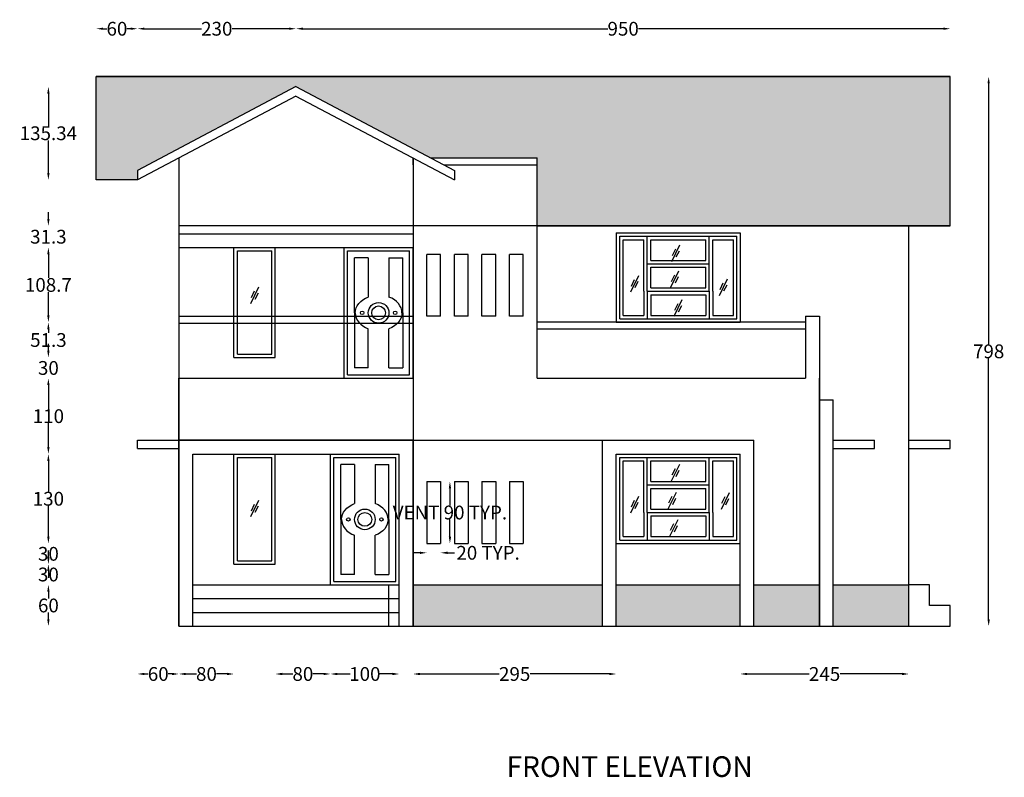
# Model space of a CAD drawing. Units: centimetres. Extents: x 10444 to 13814, y 8288 to 11191.
# Tile 1 of 9: x 10504 to 11933, y 8288 to 9388. Entities that reach past the tile are written whole.
import ezdxf

# ---------------------------------------------------------------- set-up
doc = ezdxf.new("R2010")
doc.units = ezdxf.units.CM
doc.header["$MEASUREMENT"] = 0
for name, color, linetype, lineweight in [('A-ANNO-DIMS', 2, 'Continuous', 18), ('A-ANNO-TEXT', 7, 'Continuous', 25), ('A-ELEV', 7, 'Continuous', 25), ('A-ELEV-PATT', 8, 'Continuous', 13)]:
    doc.layers.add(name, color=color, linetype=linetype, lineweight=lineweight)
doc.styles.get("Standard").update_dxf_attribs({"font": 'arial.ttf'})
doc.dimstyles.get("Standard").update_dxf_attribs({"dimtxt": 20, "dimasz": 10, "dimexe": 0.18, "dimexo": 0.0625, "dimgap": 0.09, "dimtad": 0, "dimtih": 1, "dimtoh": 1, "dimdec": 0, "dimzin": 0, "dimdsep": 46, "dimtxsty": 'Standard', "dimcen": 0.09, "dimse1": 1, "dimse2": 1, "dimadec": 0, "dimazin": 0, "dimtfac": 1, "dimtdec": 0, "dimtofl": 0, "dimtmove": 0, "dimatfit": 3, "dimfxl": 1, "dimtolj": 1, "dimtzin": 0, "dimarcsym": 0})

# ---------------------------------------------------------------- blocks, each defined once
blk = doc.blocks.new('*D26')
at = {"layer": 'A-ANNO-DIMS', "color": 0, "lineweight": -2, "transparency": 16777216}
for p, q in [((11910.5, 9295.8), (11910.5, 8917)), ((11910.5, 8517.6), (11910.5, 8896.4))]:
    blk.add_line(p, q, dxfattribs=at)
at = {"layer": 'A-ANNO-DIMS', "color": 0, "transparency": 16777216}
for points in [[(11908.8, 9295.8), (11912.2, 9295.8), (11910.5, 9305.8)], [(11908.8, 8517.6), (11912.2, 8517.6), (11910.5, 8507.6)]]:
    blk.add_solid(points, dxfattribs=at)
at = {"layer": 'Defpoints', "color": 0, "transparency": 16777216}
for p in [(11854.8, 9305.8), (11910.5, 9305.8), (11854.8, 8507.6)]:
    blk.add_point(p, dxfattribs=at)
at = {"layer": 'A-ANNO-DIMS', "color": 0, "transparency": 16777216, "insert": (11910.5, 8906.7), "char_height": 20, "attachment_point": 5}
blk.add_mtext('\\A1;798', dxfattribs=at)
blk = doc.blocks.new('ELEV-VENT')
for p, q in [((0, 90), (0, 0)), ((0, 90), (20, 90)), ((20, 90), (20, 0)), ((0, 0), (20, 0))]:
    blk.add_line(p, q)
blk = doc.blocks.new('*D49')
at = {"layer": 'A-ANNO-DIMS', "color": 0, "lineweight": -2, "transparency": 16777216}
for p, q in [((11128.3, 8707.6), (11128.3, 8682.9)), ((11128.3, 8637.6), (11128.3, 8662.3))]:
    blk.add_line(p, q, dxfattribs=at)
at = {"layer": 'A-ANNO-DIMS', "color": 0, "transparency": 16777216}
for points in [[(11126.6, 8707.6), (11130, 8707.6), (11128.3, 8717.6)], [(11126.6, 8637.6), (11130, 8637.6), (11128.3, 8627.6)]]:
    blk.add_solid(points, dxfattribs=at)
at = {"layer": 'Defpoints', "color": 0, "transparency": 16777216}
for p in [(11114.8, 8717.6), (11128.3, 8717.6), (11114.8, 8627.6)]:
    blk.add_point(p, dxfattribs=at)
at = {"layer": 'A-ANNO-DIMS', "color": 0, "transparency": 16777216, "insert": (11128.3, 8672.6), "char_height": 20, "attachment_point": 5}
blk.add_mtext('\\A1;VENT 90 TYP.', dxfattribs=at)
blk = doc.blocks.new('*D50')
at = {"layer": 'A-ANNO-DIMS', "color": 0, "lineweight": -2, "transparency": 16777216}
for p, q in [((11084.8, 8614.1), (11074.8, 8614.1)), ((11124.8, 8614.1), (11134.8, 8614.1))]:
    blk.add_line(p, q, dxfattribs=at)
at = {"layer": 'A-ANNO-DIMS', "color": 0, "transparency": 16777216}
for points in [[(11084.8, 8615.8), (11084.8, 8612.4), (11094.8, 8614.1)], [(11124.8, 8615.8), (11124.8, 8612.4), (11114.8, 8614.1)]]:
    blk.add_solid(points, dxfattribs=at)
at = {"layer": 'Defpoints', "color": 0, "transparency": 16777216}
for p in [(11094.8, 8627.6), (11114.8, 8627.6), (11114.8, 8614.1)]:
    blk.add_point(p, dxfattribs=at)
at = {"layer": 'A-ANNO-DIMS', "color": 0, "transparency": 16777216, "insert": (11183.7, 8614.1), "char_height": 20, "attachment_point": 5}
blk.add_mtext('\\A1;20 TYP.', dxfattribs=at)
blk = doc.blocks.new('*D88')
at = {"layer": 'A-ANNO-DIMS', "color": 0, "lineweight": -2, "transparency": 16777216}
for p, q in [((10624.8, 9375.3), (10630.4, 9375.3)), ((10664.8, 9375.3), (10659.2, 9375.3))]:
    blk.add_line(p, q, dxfattribs=at)
at = {"layer": 'A-ANNO-DIMS', "color": 0, "transparency": 16777216}
for points in [[(10624.8, 9377), (10624.8, 9373.7), (10614.8, 9375.3)], [(10664.8, 9377), (10664.8, 9373.7), (10674.8, 9375.3)]]:
    blk.add_solid(points, dxfattribs=at)
at = {"layer": 'Defpoints', "color": 0, "transparency": 16777216}
for p in [(10674.8, 9375.3), (10614.8, 9305.8), (10674.8, 9155.8)]:
    blk.add_point(p, dxfattribs=at)
at = {"layer": 'A-ANNO-DIMS', "color": 0, "transparency": 16777216, "insert": (10644.8, 9375.3), "char_height": 20, "attachment_point": 5}
blk.add_mtext('\\A1;60', dxfattribs=at)
blk = doc.blocks.new('*D89')
at = {"layer": 'A-ANNO-DIMS', "color": 0, "lineweight": -2, "transparency": 16777216}
for p, q in [((10684.8, 9375.3), (10767.5, 9375.3)), ((10894.8, 9375.3), (10812.1, 9375.3))]:
    blk.add_line(p, q, dxfattribs=at)
at = {"layer": 'A-ANNO-DIMS', "color": 0, "transparency": 16777216}
for points in [[(10684.8, 9377), (10684.8, 9373.7), (10674.8, 9375.3)], [(10894.8, 9377), (10894.8, 9373.7), (10904.8, 9375.3)]]:
    blk.add_solid(points, dxfattribs=at)
at = {"layer": 'Defpoints', "color": 0, "transparency": 16777216}
for p in [(10904.8, 9375.3), (10904.8, 9291.2), (10674.8, 9155.8)]:
    blk.add_point(p, dxfattribs=at)
at = {"layer": 'A-ANNO-DIMS', "color": 0, "transparency": 16777216, "insert": (10789.8, 9375.3), "char_height": 20, "attachment_point": 5}
blk.add_mtext('\\A1;230', dxfattribs=at)
blk = doc.blocks.new('*D90')
at = {"layer": 'A-ANNO-DIMS', "color": 0, "lineweight": -2, "transparency": 16777216}
for p, q in [((10914.8, 9375.3), (11357.6, 9375.3)), ((11844.8, 9375.3), (11401.9, 9375.3))]:
    blk.add_line(p, q, dxfattribs=at)
at = {"layer": 'A-ANNO-DIMS', "color": 0, "transparency": 16777216}
for points in [[(10914.8, 9377), (10914.8, 9373.7), (10904.8, 9375.3)], [(11844.8, 9377), (11844.8, 9373.7), (11854.8, 9375.3)]]:
    blk.add_solid(points, dxfattribs=at)
at = {"layer": 'Defpoints', "color": 0, "transparency": 16777216}
for p in [(11854.8, 9375.3), (11854.8, 9305.8), (10904.8, 9291.2)]:
    blk.add_point(p, dxfattribs=at)
at = {"layer": 'A-ANNO-DIMS', "color": 0, "transparency": 16777216, "insert": (11379.8, 9375.3), "char_height": 20, "attachment_point": 5}
blk.add_mtext('\\A1;950', dxfattribs=at)
blk = doc.blocks.new('*D91')
at = {"layer": 'A-ANNO-DIMS', "color": 0, "lineweight": -2, "transparency": 16777216}
for p, q in [((10684.8, 8438.1), (10690.4, 8438.1)), ((10724.8, 8438.1), (10719.2, 8438.1))]:
    blk.add_line(p, q, dxfattribs=at)
at = {"layer": 'A-ANNO-DIMS', "color": 0, "transparency": 16777216}
for points in [[(10684.8, 8439.8), (10684.8, 8436.4), (10674.8, 8438.1)], [(10724.8, 8439.8), (10724.8, 8436.4), (10734.8, 8438.1)]]:
    blk.add_solid(points, dxfattribs=at)
at = {"layer": 'Defpoints', "color": 0, "transparency": 16777216}
for p in [(10674.8, 8777.6), (10734.8, 8507.6), (10734.8, 8438.1)]:
    blk.add_point(p, dxfattribs=at)
at = {"layer": 'A-ANNO-DIMS', "color": 0, "transparency": 16777216, "insert": (10704.8, 8438.1), "char_height": 20, "attachment_point": 5}
blk.add_mtext('\\A1;60', dxfattribs=at)
blk = doc.blocks.new('*D92')
at = {"layer": 'A-ANNO-DIMS', "color": 0, "lineweight": -2, "transparency": 16777216}
for p, q in [((10744.8, 8438.1), (10760.4, 8438.1)), ((10804.8, 8438.1), (10789.2, 8438.1))]:
    blk.add_line(p, q, dxfattribs=at)
at = {"layer": 'A-ANNO-DIMS', "color": 0, "transparency": 16777216}
for points in [[(10744.8, 8439.8), (10744.8, 8436.4), (10734.8, 8438.1)], [(10804.8, 8439.8), (10804.8, 8436.4), (10814.8, 8438.1)]]:
    blk.add_solid(points, dxfattribs=at)
at = {"layer": 'Defpoints', "color": 0, "transparency": 16777216}
for p in [(10814.8, 8597.6), (10734.8, 8507.6), (10814.8, 8438.1)]:
    blk.add_point(p, dxfattribs=at)
at = {"layer": 'A-ANNO-DIMS', "color": 0, "transparency": 16777216, "insert": (10774.8, 8438.1), "char_height": 20, "attachment_point": 5}
blk.add_mtext('\\A1;80', dxfattribs=at)
blk = doc.blocks.new('*D93')
at = {"layer": 'A-ANNO-DIMS', "color": 0, "lineweight": -2, "transparency": 16777216}
for p, q in [((10884.8, 8438.1), (10900.4, 8438.1)), ((10944.8, 8438.1), (10929.2, 8438.1))]:
    blk.add_line(p, q, dxfattribs=at)
at = {"layer": 'A-ANNO-DIMS', "color": 0, "transparency": 16777216}
for points in [[(10884.8, 8439.8), (10884.8, 8436.4), (10874.8, 8438.1)], [(10944.8, 8439.8), (10944.8, 8436.4), (10954.8, 8438.1)]]:
    blk.add_solid(points, dxfattribs=at)
at = {"layer": 'Defpoints', "color": 0, "transparency": 16777216}
for p in [(10874.8, 8597.6), (10954.8, 8567.6), (10954.8, 8438.1)]:
    blk.add_point(p, dxfattribs=at)
at = {"layer": 'A-ANNO-DIMS', "color": 0, "transparency": 16777216, "insert": (10914.8, 8438.1), "char_height": 20, "attachment_point": 5}
blk.add_mtext('\\A1;80', dxfattribs=at)
blk = doc.blocks.new('*D94')
at = {"layer": 'A-ANNO-DIMS', "color": 0, "lineweight": -2, "transparency": 16777216}
for p, q in [((10964.8, 8438.1), (10983.6, 8438.1)), ((11044.8, 8438.1), (11026, 8438.1))]:
    blk.add_line(p, q, dxfattribs=at)
at = {"layer": 'A-ANNO-DIMS', "color": 0, "transparency": 16777216}
for points in [[(10964.8, 8439.8), (10964.8, 8436.4), (10954.8, 8438.1)], [(11044.8, 8439.8), (11044.8, 8436.4), (11054.8, 8438.1)]]:
    blk.add_solid(points, dxfattribs=at)
at = {"layer": 'Defpoints', "color": 0, "transparency": 16777216}
for p in [(10954.8, 8567.6), (11054.8, 8567.6), (11054.8, 8438.1)]:
    blk.add_point(p, dxfattribs=at)
at = {"layer": 'A-ANNO-DIMS', "color": 0, "transparency": 16777216, "insert": (11004.8, 8438.1), "char_height": 20, "attachment_point": 5}
blk.add_mtext('\\A1;100', dxfattribs=at)
blk = doc.blocks.new('*D95')
at = {"layer": 'A-ANNO-DIMS', "color": 0, "lineweight": -2, "transparency": 16777216}
for p, q in [((11084.8, 8438.1), (11199.9, 8438.1)), ((11359.8, 8438.1), (11244.7, 8438.1))]:
    blk.add_line(p, q, dxfattribs=at)
at = {"layer": 'A-ANNO-DIMS', "color": 0, "transparency": 16777216}
for points in [[(11084.8, 8439.8), (11084.8, 8436.4), (11074.8, 8438.1)], [(11359.8, 8439.8), (11359.8, 8436.4), (11369.8, 8438.1)]]:
    blk.add_solid(points, dxfattribs=at)
at = {"layer": 'Defpoints', "color": 0, "transparency": 16777216}
for p in [(11369.8, 8627.6), (11074.8, 8567.6), (11369.8, 8438.1)]:
    blk.add_point(p, dxfattribs=at)
at = {"layer": 'A-ANNO-DIMS', "color": 0, "transparency": 16777216, "insert": (11222.3, 8438.1), "char_height": 20, "attachment_point": 5}
blk.add_mtext('\\A1;295', dxfattribs=at)
blk = doc.blocks.new('*D96')
at = {"layer": 'A-ANNO-DIMS', "color": 0, "lineweight": -2, "transparency": 16777216}
for p, q in [((11559.8, 8438.1), (11649.9, 8438.1)), ((11784.8, 8438.1), (11694.7, 8438.1))]:
    blk.add_line(p, q, dxfattribs=at)
at = {"layer": 'A-ANNO-DIMS', "color": 0, "transparency": 16777216}
for points in [[(11559.8, 8439.8), (11559.8, 8436.4), (11549.8, 8438.1)], [(11784.8, 8439.8), (11784.8, 8436.4), (11794.8, 8438.1)]]:
    blk.add_solid(points, dxfattribs=at)
at = {"layer": 'Defpoints', "color": 0, "transparency": 16777216}
for p in [(11549.8, 8627.6), (11794.8, 8507.6), (11794.8, 8438.1)]:
    blk.add_point(p, dxfattribs=at)
at = {"layer": 'A-ANNO-DIMS', "color": 0, "transparency": 16777216, "insert": (11672.3, 8438.1), "char_height": 20, "attachment_point": 5}
blk.add_mtext('\\A1;245', dxfattribs=at)
blk = doc.blocks.new('*D97')
at = {"layer": 'A-ANNO-DIMS', "color": 0, "lineweight": -2, "transparency": 16777216}
for p, q in [((10545.3, 8557.6), (10545.3, 8547.9)), ((10545.3, 8517.6), (10545.3, 8527.3))]:
    blk.add_line(p, q, dxfattribs=at)
at = {"layer": 'A-ANNO-DIMS', "color": 0, "transparency": 16777216}
for points in [[(10543.6, 8557.6), (10547, 8557.6), (10545.3, 8567.6)], [(10543.6, 8517.6), (10547, 8517.6), (10545.3, 8507.6)]]:
    blk.add_solid(points, dxfattribs=at)
at = {"layer": 'Defpoints', "color": 0, "transparency": 16777216}
for p in [(10545.3, 8567.6), (10754.8, 8567.6), (10734.8, 8507.6)]:
    blk.add_point(p, dxfattribs=at)
at = {"layer": 'A-ANNO-DIMS', "color": 0, "transparency": 16777216, "insert": (10545.3, 8537.6), "char_height": 20, "attachment_point": 5}
blk.add_mtext('\\A1;60', dxfattribs=at)
blk = doc.blocks.new('*D98')
at = {"layer": 'A-ANNO-DIMS', "color": 0, "lineweight": -2, "transparency": 16777216}
for p, q in [((10545.3, 8607.6), (10545.3, 8617.6)), ((10545.3, 8557.6), (10545.3, 8547.6))]:
    blk.add_line(p, q, dxfattribs=at)
at = {"layer": 'A-ANNO-DIMS', "color": 0, "transparency": 16777216}
for points in [[(10543.6, 8607.6), (10547, 8607.6), (10545.3, 8597.6)], [(10543.6, 8557.6), (10547, 8557.6), (10545.3, 8567.6)]]:
    blk.add_solid(points, dxfattribs=at)
at = {"layer": 'Defpoints', "color": 0, "transparency": 16777216}
for p in [(10545.3, 8597.6), (10814.8, 8597.6), (10754.8, 8567.6)]:
    blk.add_point(p, dxfattribs=at)
at = {"layer": 'A-ANNO-DIMS', "color": 0, "transparency": 16777216, "insert": (10545.3, 8582.6), "char_height": 20, "attachment_point": 5}
blk.add_mtext('\\A1;30', dxfattribs=at)
blk = doc.blocks.new('*D99')
at = {"layer": 'A-ANNO-DIMS', "color": 0, "lineweight": -2, "transparency": 16777216}
for p, q in [((10545.3, 8637.6), (10545.3, 8647.6)), ((10545.3, 8587.6), (10545.3, 8577.6))]:
    blk.add_line(p, q, dxfattribs=at)
at = {"layer": 'A-ANNO-DIMS', "color": 0, "transparency": 16777216}
for points in [[(10543.6, 8637.6), (10547, 8637.6), (10545.3, 8627.6)], [(10543.6, 8587.6), (10547, 8587.6), (10545.3, 8597.6)]]:
    blk.add_solid(points, dxfattribs=at)
at = {"layer": 'Defpoints', "color": 0, "transparency": 16777216}
for p in [(10545.3, 8627.6), (11369.8, 8627.6), (10814.8, 8597.6)]:
    blk.add_point(p, dxfattribs=at)
at = {"layer": 'A-ANNO-DIMS', "color": 0, "transparency": 16777216, "insert": (10545.3, 8612.6), "char_height": 20, "attachment_point": 5}
blk.add_mtext('\\A1;30', dxfattribs=at)
blk = doc.blocks.new('*D100')
at = {"layer": 'A-ANNO-DIMS', "color": 0, "lineweight": -2, "transparency": 16777216}
for p, q in [((10545.3, 8747.6), (10545.3, 8702.9)), ((10545.3, 8637.6), (10545.3, 8682.3))]:
    blk.add_line(p, q, dxfattribs=at)
at = {"layer": 'A-ANNO-DIMS', "color": 0, "transparency": 16777216}
for points in [[(10543.6, 8747.6), (10547, 8747.6), (10545.3, 8757.6)], [(10543.6, 8637.6), (10547, 8637.6), (10545.3, 8627.6)]]:
    blk.add_solid(points, dxfattribs=at)
at = {"layer": 'Defpoints', "color": 0, "transparency": 16777216}
for p in [(10545.3, 8757.6), (10814.8, 8757.6), (11369.8, 8627.6)]:
    blk.add_point(p, dxfattribs=at)
at = {"layer": 'A-ANNO-DIMS', "color": 0, "transparency": 16777216, "insert": (10545.3, 8692.6), "char_height": 20, "attachment_point": 5}
blk.add_mtext('\\A1;130', dxfattribs=at)
blk = doc.blocks.new('*D101')
at = {"layer": 'A-ANNO-DIMS', "color": 0, "lineweight": -2, "transparency": 16777216}
for p, q in [((10545.3, 8857.6), (10545.3, 8822.9)), ((10545.3, 8767.6), (10545.3, 8802.3))]:
    blk.add_line(p, q, dxfattribs=at)
at = {"layer": 'A-ANNO-DIMS', "color": 0, "transparency": 16777216}
for points in [[(10543.6, 8857.6), (10547, 8857.6), (10545.3, 8867.6)], [(10543.6, 8767.6), (10547, 8767.6), (10545.3, 8757.6)]]:
    blk.add_solid(points, dxfattribs=at)
at = {"layer": 'Defpoints', "color": 0, "transparency": 16777216}
for p in [(10545.3, 8867.6), (10734.8, 8867.6), (10814.8, 8757.6)]:
    blk.add_point(p, dxfattribs=at)
at = {"layer": 'A-ANNO-DIMS', "color": 0, "transparency": 16777216, "insert": (10545.3, 8812.6), "char_height": 20, "attachment_point": 5}
blk.add_mtext('\\A1;110', dxfattribs=at)
blk = doc.blocks.new('*D102')
at = {"layer": 'A-ANNO-DIMS', "color": 0, "lineweight": -2, "transparency": 16777216}
for p, q in [((10545.3, 8907.6), (10545.3, 8917.6)), ((10545.3, 8857.6), (10545.3, 8847.6))]:
    blk.add_line(p, q, dxfattribs=at)
at = {"layer": 'A-ANNO-DIMS', "color": 0, "transparency": 16777216}
for points in [[(10543.6, 8907.6), (10547, 8907.6), (10545.3, 8897.6)], [(10543.6, 8857.6), (10547, 8857.6), (10545.3, 8867.6)]]:
    blk.add_solid(points, dxfattribs=at)
at = {"layer": 'Defpoints', "color": 0, "transparency": 16777216}
for p in [(10545.3, 8897.6), (10814.8, 8897.6), (10734.8, 8867.6)]:
    blk.add_point(p, dxfattribs=at)
at = {"layer": 'A-ANNO-DIMS', "color": 0, "transparency": 16777216, "insert": (10545.3, 8882.6), "char_height": 20, "attachment_point": 5}
blk.add_mtext('\\A1;30', dxfattribs=at)
blk = doc.blocks.new('*D103')
at = {"layer": 'A-ANNO-DIMS', "color": 0, "lineweight": -2, "transparency": 16777216}
for p, q in [((10545.3, 8938.9), (10545.3, 8933.6)), ((10545.3, 8907.6), (10545.3, 8912.9))]:
    blk.add_line(p, q, dxfattribs=at)
at = {"layer": 'A-ANNO-DIMS', "color": 0, "transparency": 16777216}
for points in [[(10543.6, 8938.9), (10547, 8938.9), (10545.3, 8948.9)], [(10543.6, 8907.6), (10547, 8907.6), (10545.3, 8897.6)]]:
    blk.add_solid(points, dxfattribs=at)
at = {"layer": 'Defpoints', "color": 0, "transparency": 16777216}
for p in [(10545.3, 8948.9), (11369.8, 8948.9), (10814.8, 8897.6)]:
    blk.add_point(p, dxfattribs=at)
at = {"layer": 'A-ANNO-DIMS', "color": 0, "transparency": 16777216, "insert": (10545.3, 8923.2), "char_height": 20, "attachment_point": 5}
blk.add_mtext('\\A1;51.3', dxfattribs=at)
blk = doc.blocks.new('*D104')
at = {"layer": 'A-ANNO-DIMS', "color": 0, "lineweight": -2, "transparency": 16777216}
for p, q in [((10545.3, 9047.6), (10545.3, 9013.5)), ((10545.3, 8958.9), (10545.3, 8992.9))]:
    blk.add_line(p, q, dxfattribs=at)
at = {"layer": 'A-ANNO-DIMS', "color": 0, "transparency": 16777216}
for points in [[(10543.6, 9047.6), (10547, 9047.6), (10545.3, 9057.6)], [(10543.6, 8958.9), (10547, 8958.9), (10545.3, 8948.9)]]:
    blk.add_solid(points, dxfattribs=at)
at = {"layer": 'Defpoints', "color": 0, "transparency": 16777216}
for p in [(10545.3, 9057.6), (10814.8, 9057.6), (11369.8, 8948.9)]:
    blk.add_point(p, dxfattribs=at)
at = {"layer": 'A-ANNO-DIMS', "color": 0, "transparency": 16777216, "insert": (10545.3, 9003.2), "char_height": 20, "attachment_point": 5}
blk.add_mtext('\\A1;108.7', dxfattribs=at)
blk = doc.blocks.new('*D105')
at = {"layer": 'A-ANNO-DIMS', "color": 0, "lineweight": -2, "transparency": 16777216}
for p, q in [((10545.3, 9098.9), (10545.3, 9108.9)), ((10545.3, 9047.6), (10545.3, 9037.6))]:
    blk.add_line(p, q, dxfattribs=at)
at = {"layer": 'A-ANNO-DIMS', "color": 0, "transparency": 16777216}
for points in [[(10543.6, 9098.9), (10547, 9098.9), (10545.3, 9088.9)], [(10543.6, 9047.6), (10547, 9047.6), (10545.3, 9057.6)]]:
    blk.add_solid(points, dxfattribs=at)
at = {"layer": 'Defpoints', "color": 0, "transparency": 16777216}
for p in [(10545.3, 9088.9), (11854.8, 9088.9), (10814.8, 9057.6)]:
    blk.add_point(p, dxfattribs=at)
at = {"layer": 'A-ANNO-DIMS', "color": 0, "transparency": 16777216, "insert": (10545.3, 9073.2), "char_height": 20, "attachment_point": 5}
blk.add_mtext('\\A1;31.3', dxfattribs=at)
blk = doc.blocks.new('*D106')
at = {"layer": 'A-ANNO-DIMS', "color": 0, "lineweight": -2, "transparency": 16777216}
for p, q in [((10545.3, 9281.2), (10545.3, 9233.8)), ((10545.3, 9165.8), (10545.3, 9213.2))]:
    blk.add_line(p, q, dxfattribs=at)
at = {"layer": 'A-ANNO-DIMS', "color": 0, "transparency": 16777216}
for points in [[(10543.6, 9281.2), (10547, 9281.2), (10545.3, 9291.2)], [(10543.6, 9165.8), (10547, 9165.8), (10545.3, 9155.8)]]:
    blk.add_solid(points, dxfattribs=at)
at = {"layer": 'Defpoints', "color": 0, "transparency": 16777216}
for p in [(10545.3, 9291.2), (10904.8, 9291.2), (10674.8, 9155.8)]:
    blk.add_point(p, dxfattribs=at)
at = {"layer": 'A-ANNO-DIMS', "color": 0, "transparency": 16777216, "insert": (10545.3, 9223.5), "char_height": 20, "attachment_point": 5}
blk.add_mtext('\\A1;135.34', dxfattribs=at)

msp = doc.modelspace()

# ---------------------------------------------------------------- hatches: boundary and pattern name
at = {"layer": 'A-ELEV-PATT'}
h = msp.add_hatch(dxfattribs=at)
h.set_pattern_fill('CORK', color=256, scale=40)
h.set_pattern_definition([(0, (0, 0), (0, 5), []), (135, (2.5, -2.5), (-10, -10), [7.071068, -7.071068]), (135, (3.75, -2.5), (-10, -10), [7.071068, -7.071068]), (135, (5, -2.5), (-10, -10), [7.071068, -7.071068])])
h.paths.add_polyline_path([(11854.7881, 9305.8312), (10614.7881, 9305.8312), (10614.7881, 9155.8312), (10674.7881, 9155.8312), (10674.7881, 9169.4091), (10904.7881, 9291.1738), (11100.4353, 9187.5959), (11254.7881, 9187.5959), (11254.7881, 9088.8963), (11854.7881, 9088.8963)])
h = msp.add_hatch(dxfattribs=at)
h.set_pattern_fill('GRAVEL', color=256, scale=39)
h.set_pattern_definition([(228.012788, (28.08, 39), (-312, -351), [5.2469, -519.44443]), (184.969741, (24.57, 35.1), (468, 39), [9.00385, -891.38107]), (132.510447, (15.6, 34.32), (390, -429), [6.34873, -628.52527]), (267.273689, (0.39, 24.57), (39, 780), [8.19928, -811.72876]), (292.833654, (0, 16.38), (-195, 468), [8.040045, -795.96555]), (357.273689, (3.12, 8.97), (-780, 39), [8.19928, -811.72876]), (37.69424, (11.31, 8.58), (-507, -390), [10.84313, -1073.46909]), (72.255328, (19.89, 15.21), (273, 858), [10.23703, -1013.46654]), (121.429566, (23.01, 24.96), (-312, 507), [8.22705, -814.47885]), (175.236358, (18.72, 31.98), (429, -39), [9.39245, -460.22974]), (222.397438, (9.36, 32.76), (-468, -429), [12.14647, -1202.50163]), (138.814075, (39, 24.18), (-273, 234), [4.14574, -410.42995]), (171.469234, (35.88, 26.91), (507, -78), [7.88724, -780.83895]), (225, (28.08, 28.08), (-4e-15, -39), [5.51542, -49.63891]), (203.19859, (25.35, 32.76), (195, 78), [2.97016, -294.04499]), (291.80141, (22.62, 31.59), (-39, 117), [4.20042, -205.82101]), (30.963757, (24.18, 27.69), (117, 78), [6.82223, -220.58489]), (161.56505, (30.03, 31.2), (78, -39), [4.93315, -118.39568]), (16.38954, (0, 31.59), (390, 117), [6.9108, -684.17096]), (70.346176, (6.63, 33.54), (-156, -429), [5.79778, -573.9789]), (293.19859, (30.03, 39), (-78, 195), [5.94029, -291.07487]), (343.61046, (32.37, 33.54), (-390, 117), [6.9108, -684.17096]), (339.443955, (0, 7.41), (-195, 78), [6.66432, -326.55183]), (294.77514, (6.24, 5.07), (-195, 429), [5.58394, -552.81108]), (66.80141, (30.42, 0), (78, 195), [5.94029, -291.07487]), (17.354025, (32.76, 5.46), (-507, -156), [6.53761, -647.22152]), (69.443955, (11.31, 0), (-78, -195), [3.33216, -329.88399]), (101.30993, (28.08, 0), (-39, 156), [1.98861, -196.87315]), (165.96376, (27.69, 1.95), (117, -39), [8.04004, -152.76107]), (186.009006, (19.89, 3.9), (390, 39), [7.45095, -737.643]), (303.69007, (24.18, 24.18), (-39, 78), [5.62466, -134.99184]), (353.157227, (27.3, 19.5), (663, -78), [9.81997, -972.17494]), (60.945396, (37.05, 18.33), (-156, -273), [4.01528, -397.51429]), (90, (39, 21.84), (-39, 39), [2.34, -36.66]), (120.256437, (19.11, 5.07), (156, -273), [5.41804, -536.38728]), (48.012788, (16.38, 9.75), (312, 351), [10.49381, -514.19753]), (0, (23.4, 17.55), (39, 39), [10.14, -28.86]), (325.304846, (33.54, 17.55), (390, -273), [6.16645, -610.4777]), (254.054604, (38.61, 14.04), (-39, -156), [5.67848, -278.24581]), (207.645975, (37.05, 8.58), (-741, -390), [9.245535, -915.30949]), (175.426079, (28.86, 4.29), (-507, 39), [9.78116, -968.33386])])
h.paths.add_polyline_path([(11349.7881, 8567.5959), (11074.7881, 8567.5959), (11074.7881, 8507.5959), (11349.7881, 8507.5959)])
h.paths.add_polyline_path([(11549.7881, 8567.5959), (11369.7881, 8567.5959), (11369.7881, 8507.5959), (11549.7881, 8507.5959)])
h.paths.add_polyline_path([(11664.7881, 8567.5959), (11569.7881, 8567.5959), (11569.7881, 8507.5959), (11664.7881, 8507.5959)])
h.paths.add_polyline_path([(11794.7881, 8567.5959), (11684.7881, 8567.5959), (11684.7881, 8507.5959), (11794.7881, 8507.5959)])

# ---------------------------------------------------------------- linework, layer by layer
at = {"layer": 'A-ELEV'}
for p, q in [((10614.7881, 9155.8312), (10614.7881, 9305.8312)), ((10674.7881, 9305.8312), (10614.7881, 9305.8312)), ((10614.7881, 9305.8312), (11854.7881, 9305.8312)), ((11854.7881, 9305.8312), (10614.7881, 9305.8312)), ((11854.7881, 9088.8963), (11854.7881, 9305.8312)), ((10904.7881, 9291.1738), (10674.7881, 9169.4091)), ((10904.7881, 9291.1738), (11134.7881, 9169.4091)), ((10904.7881, 9277.5959), (10674.7881, 9155.8312)), ((10904.7881, 9277.5959), (11134.7881, 9155.8312)), ((10734.7881, 9187.5959), (10734.7881, 8507.5959)), ((10734.7881, 9187.5959), (10734.7881, 8507.5959)), ((11074.7881, 9177.5959), (11074.7881, 9187.5959)), ((11074.7881, 9187.5959), (11074.7881, 8507.5959)), ((11100.4353, 9187.5959), (11254.7881, 9187.5959)), ((11254.7881, 8867.5959), (11254.7881, 9187.5959)), ((10674.7881, 9169.4091), (10674.7881, 9155.8312)), ((11119.3242, 9177.5959), (11254.7881, 9177.5959)), ((11134.7881, 9169.4091), (11134.7881, 9155.8312)), ((10674.7881, 9155.8312), (10614.7881, 9155.8312)), ((10674.7881, 9155.8312), (10614.7881, 9155.8312)), ((11854.7881, 9088.8963), (10734.7881, 9088.8963)), ((11254.7881, 9088.8963), (11854.7881, 9088.8963)), ((11369.7881, 9078.8963), (11549.7881, 9078.8963)), ((11369.7881, 9078.8963), (11369.7881, 8948.8963)), ((11549.7881, 9078.8963), (11549.7881, 8948.8963)), ((11794.7881, 8507.5959), (11794.7881, 9088.8963)), ((10734.7881, 9077.5959), (11074.7881, 9077.5959)), ((11374.7881, 8953.8963), (11374.7881, 9073.8963)), ((11374.7881, 9073.8963), (11544.7881, 9073.8963)), ((11379.7881, 8958.8963), (11379.7881, 9068.8963)), ((11379.7881, 9068.8963), (11409.7881, 9068.8963)), ((11409.7881, 9033.8963), (11409.7881, 9068.8963)), ((11414.7881, 9033.8963), (11414.7881, 9073.8963)), ((11419.7881, 9068.8963), (11499.7881, 9068.8963)), ((11419.7881, 9038.8963), (11419.7881, 9068.8963)), ((11499.7881, 9038.8963), (11499.7881, 9068.8963)), ((11504.7881, 9033.8963), (11504.7881, 9073.8963)), ((11509.7881, 9068.8963), (11539.7881, 9068.8963)), ((11509.7881, 9033.8963), (11509.7881, 9068.8963)), ((11539.7881, 8958.8963), (11539.7881, 9068.8963)), ((11544.7881, 8953.8963), (11544.7881, 9073.8963)), ((10734.7881, 9057.5959), (11074.7881, 9057.5959)), ((10814.7881, 8897.5959), (10814.7881, 9057.5959)), ((10819.7881, 9052.5959), (10869.7881, 9052.5959)), ((10819.7881, 8902.5959), (10819.7881, 9052.5959)), ((10869.7881, 8902.5959), (10869.7881, 9052.5959)), ((10874.7881, 8897.5959), (10874.7881, 9057.5959)), ((10974.7881, 9057.5959), (11074.7881, 9057.5959)), ((10974.7881, 8867.5959), (10974.7881, 9057.5959)), ((10979.7881, 8872.5959), (10979.7881, 9052.5959)), ((10979.7881, 9052.5959), (11069.7881, 9052.5959)), ((11069.7881, 8872.5959), (11069.7881, 9052.5959)), ((11074.7881, 8867.5959), (11074.7881, 9057.5959)), ((11461.7732, 9060.9147), (11450.0244, 9036.8125)), ((11455.5852, 9055.0669), (11450.8854, 9045.4254)), ((11460.9747, 9052.4299), (11456.5226, 9043.2967)), ((10989.7881, 8962.5959), (10989.7881, 9042.5959)), ((11009.7881, 9042.5959), (10989.7881, 9042.5959)), ((11009.7881, 9042.5959), (11009.7881, 8985.6497)), ((11039.7881, 9042.5959), (11059.7881, 9042.5959)), ((11039.7881, 9042.5959), (11039.7881, 8985.6497)), ((11059.7881, 8962.5959), (11059.7881, 9042.5959)), ((11419.7881, 9038.8963), (11499.7881, 9038.8963)), ((11409.7881, 8993.8963), (11409.7881, 9033.8963)), ((11414.7881, 8993.8963), (11414.7881, 9033.8963)), ((11414.7881, 9033.8963), (11504.7881, 9033.8963)), ((11419.7881, 8998.8963), (11419.7881, 9028.8963)), ((11419.7881, 9028.8963), (11499.7881, 9028.8963)), ((11460.3527, 9023.3751), (11448.604, 8999.2729)), ((11499.7881, 8998.8963), (11499.7881, 9028.8963)), ((11504.7881, 8993.8963), (11504.7881, 9033.8963)), ((11509.7881, 8993.8963), (11509.7881, 9033.8963)), ((11402.1658, 9016.5745), (11390.417, 8992.4723)), ((11395.9778, 9010.7266), (11391.278, 9001.0851)), ((11401.3672, 9008.0897), (11396.9152, 8998.9565)), ((11454.1647, 9017.5272), (11449.4649, 9007.8857)), ((11459.5542, 9014.8903), (11455.1021, 9005.7571)), ((11530.931, 9011.5139), (11519.1823, 8987.4117)), ((10850.4562, 8999.74), (10838.7075, 8975.6378)), ((10844.2682, 8993.8921), (10839.5684, 8984.2506)), ((11409.7881, 8993.8963), (11409.7881, 8958.8963)), ((11414.7881, 8993.8963), (11504.7881, 8993.8963)), ((11414.7881, 8993.8963), (11414.7881, 8953.8963)), ((11419.7881, 8998.8963), (11499.7881, 8998.8963)), ((11504.7881, 8993.8963), (11504.7881, 8953.8963)), ((11509.7881, 8993.8963), (11509.7881, 8958.8963)), ((11524.743, 9005.666), (11520.0432, 8996.0245)), ((11530.1325, 9003.029), (11525.6805, 8993.8959)), ((10849.6577, 8991.2552), (10845.2057, 8982.122)), ((11419.7881, 8988.8963), (11499.7881, 8988.8963)), ((11419.7881, 8988.8963), (11419.7881, 8958.8963)), ((11465.1781, 8981.4131), (11453.4294, 8957.3109)), ((11499.7881, 8988.8963), (11499.7881, 8958.8963)), ((11458.9901, 8975.5652), (11454.2903, 8965.9237)), ((11464.3796, 8972.9283), (11459.9275, 8963.7951)), ((10734.7881, 8957.5959), (11074.7881, 8957.5959)), ((10989.7881, 8962.5959), (10989.7881, 8882.5959)), ((11058.6936, 8962.5959), (11059.7881, 8962.5959)), ((11059.7881, 8962.5959), (11059.7881, 8882.5959)), ((11374.7881, 8953.8963), (11544.7881, 8953.8963)), ((11379.7881, 8958.8963), (11409.7881, 8958.8963)), ((11419.7881, 8958.8963), (11499.7881, 8958.8963)), ((11509.7881, 8958.8963), (11539.7881, 8958.8963)), ((11644.7881, 8957.5959), (11644.7881, 8867.5959)), ((11644.7881, 8957.5959), (11664.7881, 8957.5959)), ((11664.7881, 8957.5959), (11664.7881, 8507.5959)), ((10734.7881, 8947.5959), (11074.7881, 8947.5959)), ((11009.7881, 8882.5959), (11009.7881, 8939.5421)), ((11039.7881, 8882.5959), (11039.7881, 8939.5421)), ((11644.7881, 8948.8963), (11254.7881, 8948.8963)), ((11644.7881, 8938.8963), (11254.7881, 8938.8963)), ((11369.7881, 8948.8963), (11549.7881, 8948.8963)), ((10814.7881, 8897.5959), (10874.7881, 8897.5959)), ((10819.7881, 8902.5959), (10869.7881, 8902.5959)), ((11009.7881, 8882.5959), (10989.7881, 8882.5959)), ((11039.7881, 8882.5959), (11059.7881, 8882.5959)), ((10734.7881, 8507.5959), (10734.7881, 8867.5959)), ((10734.7881, 8867.5959), (11074.7881, 8867.5959)), ((10974.7881, 8867.5959), (11074.7881, 8867.5959)), ((10979.7881, 8872.5959), (11069.7881, 8872.5959)), ((11074.7881, 8867.5959), (11074.7881, 8877.5959)), ((11254.7881, 8867.5959), (11644.7881, 8867.5959)), ((11664.7881, 8507.5959), (11664.7881, 8867.5959)), ((11664.7881, 8836.4833), (11684.7881, 8836.4833)), ((11684.7881, 8507.5959), (11684.7881, 8836.4833)), ((10674.7881, 8777.5959), (11569.7881, 8777.5959)), ((10674.7881, 8765.5959), (10674.7881, 8777.5959)), ((10674.7881, 8765.5959), (10734.7881, 8765.5959)), ((11074.7881, 8777.5959), (10734.7881, 8777.5959)), ((11074.7881, 8507.5959), (11074.7881, 8777.5959)), ((11074.7881, 8777.5959), (11074.7881, 8507.5959)), ((11349.7881, 8777.5959), (11569.7881, 8777.5959)), ((11349.7881, 8507.5959), (11349.7881, 8777.5959)), ((11569.7881, 8507.5959), (11569.7881, 8777.5959)), ((11684.7881, 8777.5959), (11744.7881, 8777.5959)), ((11684.7881, 8765.5959), (11744.7881, 8765.5959)), ((11744.7881, 8765.5959), (11744.7881, 8777.5959)), ((11794.7881, 8777.5959), (11854.7881, 8777.5959)), ((11794.7881, 8765.5959), (11854.7881, 8765.5959)), ((11854.7881, 8765.5959), (11854.7881, 8777.5959)), ((11854.7881, 8765.5959), (11854.7881, 8777.5959)), ((10754.7881, 8757.5959), (11054.7881, 8757.5959)), ((10754.7881, 8507.5959), (10754.7881, 8757.5959)), ((10814.7881, 8597.5959), (10814.7881, 8757.5959)), ((10819.7881, 8602.5959), (10819.7881, 8752.5959)), ((10819.7881, 8752.5959), (10869.7881, 8752.5959)), ((10869.7881, 8602.5959), (10869.7881, 8752.5959)), ((10874.7881, 8597.5959), (10874.7881, 8757.5959)), ((10954.7881, 8567.5959), (10954.7881, 8757.5959)), ((10954.7881, 8757.5959), (11054.7881, 8757.5959)), ((10959.7881, 8752.5959), (11049.7881, 8752.5959)), ((10959.7881, 8572.5959), (10959.7881, 8752.5959)), ((11049.7881, 8572.5959), (11049.7881, 8752.5959)), ((11054.7881, 8507.5959), (11054.7881, 8757.5959)), ((11369.7881, 8507.5959), (11369.7881, 8757.5959)), ((11369.7881, 8757.5959), (11549.7881, 8757.5959)), ((11374.7881, 8752.5959), (11544.7881, 8752.5959)), ((11374.7881, 8632.5959), (11374.7881, 8752.5959)), ((11414.7881, 8712.5959), (11414.7881, 8752.5959)), ((11504.7881, 8712.5959), (11504.7881, 8752.5959)), ((11544.7881, 8632.5959), (11544.7881, 8752.5959)), ((11549.7881, 8507.5959), (11549.7881, 8757.5959)), ((10969.7881, 8662.5959), (10969.7881, 8742.5959)), ((10989.7881, 8742.5959), (10969.7881, 8742.5959)), ((10989.7881, 8742.5959), (10989.7881, 8685.6497)), ((11019.7881, 8742.5959), (11019.7881, 8685.6497)), ((11019.7881, 8742.5959), (11039.7881, 8742.5959)), ((11039.7881, 8662.5959), (11039.7881, 8742.5959)), ((11379.7881, 8747.5959), (11409.7881, 8747.5959)), ((11379.7881, 8637.5959), (11379.7881, 8747.5959)), ((11409.7881, 8712.5959), (11409.7881, 8747.5959)), ((11419.7881, 8717.5959), (11419.7881, 8747.5959)), ((11419.7881, 8747.5959), (11499.7881, 8747.5959)), ((11461.4162, 8742.1319), (11449.6675, 8718.0297)), ((11455.2282, 8736.284), (11450.5284, 8726.6425)), ((11499.7881, 8717.5959), (11499.7881, 8747.5959)), ((11509.7881, 8747.5959), (11539.7881, 8747.5959)), ((11509.7881, 8712.5959), (11509.7881, 8747.5959)), ((11539.7881, 8637.5959), (11539.7881, 8747.5959)), ((11460.6177, 8733.6471), (11456.1657, 8724.5139)), ((11409.7881, 8672.5959), (11409.7881, 8712.5959)), ((11414.7881, 8712.5959), (11504.7881, 8712.5959)), ((11414.7881, 8672.5959), (11414.7881, 8712.5959)), ((11419.7881, 8717.5959), (11499.7881, 8717.5959)), ((11419.7881, 8707.5959), (11499.7881, 8707.5959)), ((11419.7881, 8677.5959), (11419.7881, 8707.5959)), ((11499.7881, 8677.5959), (11499.7881, 8707.5959)), ((11504.7881, 8672.5959), (11504.7881, 8712.5959)), ((11509.7881, 8672.5959), (11509.7881, 8712.5959)), ((11402.1157, 8695.7649), (11390.3669, 8671.6628)), ((11456.6339, 8701.501), (11444.8852, 8677.3988)), ((11450.4459, 8695.6532), (11445.7461, 8686.0117)), ((11455.8354, 8693.0162), (11451.3834, 8683.883)), ((11533.6289, 8701.023), (11521.8801, 8676.9209)), ((11527.4409, 8695.1752), (11522.741, 8685.5337)), ((11532.8303, 8692.5382), (11528.3783, 8683.405)), ((10850.4562, 8690.2419), (10838.7075, 8666.1398)), ((10844.2682, 8684.3941), (10839.5684, 8674.7526)), ((10849.6577, 8681.7571), (10845.2057, 8672.6239)), ((11395.9277, 8689.9171), (11391.2279, 8680.2756)), ((11401.3172, 8687.2801), (11396.8651, 8678.1469)), ((11419.7881, 8677.5959), (11499.7881, 8677.5959)), ((11409.7881, 8672.5959), (11409.7881, 8637.5959)), ((11414.7881, 8672.5959), (11504.7881, 8672.5959)), ((11414.7881, 8672.5959), (11414.7881, 8632.5959)), ((11419.7881, 8667.5959), (11499.7881, 8667.5959)), ((11419.7881, 8667.5959), (11419.7881, 8637.5959)), ((11499.7881, 8667.5959), (11499.7881, 8637.5959)), ((11504.7881, 8672.5959), (11504.7881, 8632.5959)), ((11509.7881, 8672.5959), (11509.7881, 8637.5959)), ((10969.7881, 8662.5959), (10969.7881, 8582.5959)), ((11038.6936, 8662.5959), (11039.7881, 8662.5959)), ((11039.7881, 8662.5959), (11039.7881, 8582.5959)), ((11459.0251, 8661.8262), (11447.2763, 8637.724)), ((11452.8371, 8655.9784), (11448.1373, 8646.3369)), ((11458.2266, 8653.3414), (11453.7745, 8644.2082)), ((10989.7881, 8582.5959), (10989.7881, 8639.5421)), ((11019.7881, 8582.5959), (11019.7881, 8639.5421)), ((11379.7881, 8637.5959), (11409.7881, 8637.5959)), ((11419.7881, 8637.5959), (11499.7881, 8637.5959)), ((11509.7881, 8637.5959), (11539.7881, 8637.5959)), ((11369.7881, 8627.5959), (11549.7881, 8627.5959)), ((11374.7881, 8632.5959), (11544.7881, 8632.5959)), ((10814.7881, 8597.5959), (10874.7881, 8597.5959)), ((10819.7881, 8602.5959), (10869.7881, 8602.5959)), ((10989.7881, 8582.5959), (10969.7881, 8582.5959)), ((11019.7881, 8582.5959), (11039.7881, 8582.5959)), ((10754.7881, 8567.5959), (11054.7881, 8567.5959)), ((10959.7881, 8572.5959), (11049.7881, 8572.5959)), ((11039.7881, 8507.5959), (11039.7881, 8567.5959)), ((11074.7881, 8567.5959), (11349.7881, 8567.5959)), ((11369.7881, 8567.5959), (11549.7881, 8567.5959)), ((11569.7881, 8567.5959), (11664.7881, 8567.5959)), ((11684.7881, 8567.5959), (11794.7881, 8567.5959)), ((11824.7881, 8567.5959), (11794.7881, 8567.5959)), ((11824.7881, 8537.5959), (11824.7881, 8567.5959)), ((10754.7881, 8547.5959), (11054.7881, 8547.5959)), ((11854.7881, 8537.5959), (11824.7881, 8537.5959)), ((11854.7881, 8507.5959), (11854.7881, 8537.5959)), ((10754.7881, 8527.5959), (11054.7881, 8527.5959)), ((10734.7881, 8507.5959), (11794.7881, 8507.5959)), ((11794.7881, 8507.5959), (11854.7881, 8507.5959))]:
    msp.add_line(p, q, dxfattribs=at)
for centre, radius in [((11000.8406, 8962.5959), 2.5), ((11024.7881, 8962.5959), 15), ((11024.7881, 8962.5959), 10), ((11048.8092, 8962.5959), 2.5), ((11004.7881, 8662.5959), 15), ((10980.8406, 8662.5959), 2.5), ((11004.7881, 8662.5959), 10), ((11028.8092, 8662.5959), 2.5)]:
    msp.add_circle(centre, radius, dxfattribs=at)
at = {"layer": 'A-ELEV', "extrusion": (0, 0, -1)}
for centre, major_axis in [((11024.7881, 8962.5959), (-33.9055, 0)), ((11024.7881, 8962.5959), (33.9055, 0)), ((11004.7881, 8662.5959), (-33.9055, 0)), ((11004.7881, 8662.5959), (33.9055, 0))]:
    msp.add_ellipse(centre, major_axis=major_axis, ratio=0.758174406, start_param=6.283185307, end_param=7.395701894, dxfattribs=at)
at = {"layer": 'A-ELEV'}
for centre, major_axis in [((11024.7881, 8962.5959), (33.9055, 0)), ((11024.7881, 8962.5959), (-33.9055, 0)), ((11004.7881, 8662.5959), (33.9055, 0)), ((11004.7881, 8662.5959), (-33.9055, 0))]:
    msp.add_ellipse(centre, major_axis=major_axis, ratio=0.758174406, start_param=6.283185307, end_param=7.395701894, dxfattribs=at)

# ---------------------------------------------------------------- block references
at = {"layer": 'A-ELEV', "rotation": 180}
for p in [(11114.7882, 9047.5958), (11154.7882, 9047.5958), (11194.7882, 9047.5958), (11234.7882, 9047.5958)]:
    msp.add_blockref('ELEV-VENT', p, dxfattribs=at)
at = {"layer": 'A-ELEV'}
for p in [(11094.788, 8627.596), (11134.788, 8627.596), (11174.788, 8627.596), (11214.788, 8627.596)]:
    msp.add_blockref('ELEV-VENT', p, dxfattribs=at)

# ---------------------------------------------------------------- texts
at = {"layer": 'A-ANNO-TEXT', "insert": (11073, 8318.5437), "char_height": 30, "attachment_point": 1}
msp.add_mtext_dynamic_manual_height_columns('\\pxqc;FRONT ELEVATION', width=632.311628, gutter_width=1, heights=[20.6958], dxfattribs=at)

# ---------------------------------------------------------------- dimensions: what is measured, and where the dimension line sits
at = {"layer": 'A-ANNO-DIMS'}
for base, p1, p2, picture, middle in [((10674.7881, 9375.3312), (10614.7881, 9305.8312), (10674.7881, 9155.8312), '*D88', (10644.7881, 9375.3312)), ((10904.7881, 9375.3312), (10674.7881, 9155.8312), (10904.7881, 9291.1738), '*D89', (10789.7881, 9375.3312)), ((11854.7881, 9375.3312), (10904.7881, 9291.1738), (11854.7881, 9305.8312), '*D90', (11379.7881, 9375.3312)), ((10734.7881, 8438.0959), (10674.7881, 8777.5959), (10734.7881, 8507.5959), '*D91', (10704.7881, 8438.0959)), ((11369.7881, 8438.0959), (11074.7881, 8567.5959), (11369.7881, 8627.5959), '*D95', (11222.2881, 8438.0959)), ((11794.7881, 8438.0959), (11549.7881, 8627.5959), (11794.7881, 8507.5959), '*D96', (11672.2881, 8438.0959)), ((10814.7881, 8438.0959), (10734.7881, 8507.5959), (10814.7881, 8597.5959), '*D92', (10774.7881, 8438.0959)), ((10954.7881, 8438.0959), (10874.7881, 8597.5959), (10954.7881, 8567.5959), '*D93', (10914.7881, 8438.0959)), ((11054.7881, 8438.0959), (10954.7881, 8567.5959), (11054.7881, 8567.5959), '*D94', (11004.7881, 8438.0959))]:
    dim = msp.add_linear_dim(base=base, p1=p1, p2=p2, dimstyle='Standard', override={"dimdec": 0, "dimlfac": 1, "dimrnd": 0, "dimzin": 0, "dimdsep": 46, "dimlunit": 2}, dxfattribs=at)
    dim.commit()
    dim.dimension.update_dxf_attribs({"geometry": picture, "text_midpoint": middle})
dim = msp.add_aligned_dim(p1=(11854.7881, 8507.5959), p2=(11854.7881, 9305.8312), distance=-55.7119, dimstyle='Standard', override={"dimclrd": 0, "dimclre": 0, "dimclrt": 0}, dxfattribs=at)
dim.commit()
dim.dimension.update_dxf_attribs({"geometry": '*D26', "text_midpoint": (11910.5, 8906.7136)})
for base, p1, p2, override, picture, middle in [((10545.2881, 9291.1738), (10674.7881, 9155.8312), (10904.7881, 9291.1738), {"dimdec": 2, "dimlfac": 1, "dimrnd": 0, "dimzin": 0, "dimdsep": 46, "dimlunit": 2}, '*D106', (10545.2881, 9223.5025)), ((10545.2881, 9088.8963), (10814.7881, 9057.5959), (11854.7881, 9088.8963), {"dimdec": 1, "dimlfac": 1, "dimrnd": 0, "dimzin": 0, "dimdsep": 46, "dimlunit": 2}, '*D105', (10545.2881, 9073.2461)), ((10545.2881, 9057.5959), (11369.7881, 8948.8963), (10814.7881, 9057.5959), {"dimdec": 1, "dimlfac": 1, "dimrnd": 0, "dimzin": 0, "dimdsep": 46, "dimlunit": 2}, '*D104', (10545.2881, 9003.2461)), ((10545.2881, 8948.8963), (10814.7881, 8897.5959), (11369.7881, 8948.8963), {"dimdec": 1, "dimlfac": 1, "dimrnd": 0, "dimzin": 0, "dimdsep": 46, "dimlunit": 2}, '*D103', (10545.2881, 8923.2461)), ((10545.2881, 8897.5959), (10734.7881, 8867.5959), (10814.7881, 8897.5959), {"dimdec": 0, "dimlfac": 1, "dimrnd": 0, "dimzin": 0, "dimdsep": 46, "dimlunit": 2}, '*D102', (10545.2881, 8882.5959)), ((10545.2881, 8867.5959), (10814.7881, 8757.5959), (10734.7881, 8867.5959), {"dimdec": 0, "dimlfac": 1, "dimrnd": 0, "dimzin": 0, "dimdsep": 46, "dimlunit": 2}, '*D101', (10545.2881, 8812.5959)), ((10545.2881, 8757.5959), (11369.7881, 8627.5959), (10814.7881, 8757.5959), {"dimdec": 0, "dimlfac": 1, "dimrnd": 0, "dimzin": 0, "dimdsep": 46, "dimlunit": 2}, '*D100', (10545.2881, 8692.5959)), ((10545.2881, 8627.5959), (10814.7881, 8597.5959), (11369.7881, 8627.5959), {"dimdec": 0, "dimlfac": 1, "dimrnd": 0, "dimzin": 0, "dimdsep": 46, "dimlunit": 2}, '*D99', (10545.2881, 8612.5959)), ((10545.2881, 8597.5959), (10754.7881, 8567.5959), (10814.7881, 8597.5959), {"dimdec": 0, "dimlfac": 1, "dimrnd": 0, "dimzin": 0, "dimdsep": 46, "dimlunit": 2}, '*D98', (10545.2881, 8582.5959)), ((10545.2881, 8567.5959), (10734.7881, 8507.5959), (10754.7881, 8567.5959), {"dimdec": 0, "dimlfac": 1, "dimrnd": 0, "dimzin": 0, "dimdsep": 46, "dimlunit": 2}, '*D97', (10545.2881, 8537.5959))]:
    dim = msp.add_linear_dim(base=base, p1=p1, p2=p2, angle=90, dimstyle='Standard', override=override, dxfattribs=at)
    dim.commit()
    dim.dimension.update_dxf_attribs({"geometry": picture, "text_midpoint": middle})
dim = msp.add_linear_dim(base=(11128.2881, 8717.5959), p1=(11114.7881, 8627.5959), p2=(11114.7881, 8717.5959), angle=90, text='VENT <> TYP.', dimstyle='Standard', override={"dimdec": 0, "dimrnd": 0, "dimzin": 0, "dimlunit": 2}, dxfattribs=at)
dim.commit()
dim.dimension.update_dxf_attribs({"geometry": '*D49', "text_midpoint": (11128.2881, 8672.5959)})
dim = msp.add_linear_dim(base=(11114.7881, 8614.0959), p1=(11094.7881, 8627.5959), p2=(11114.7881, 8627.5959), text='<> TYP.', dimstyle='Standard', override={"dimdec": 0, "dimrnd": 0, "dimzin": 0, "dimlunit": 2}, dxfattribs=at)
dim.commit()
dim.dimension.update_dxf_attribs({"geometry": '*D50', "text_midpoint": (11183.7253, 8614.0959)})

doc.saveas('drawing.dxf')
